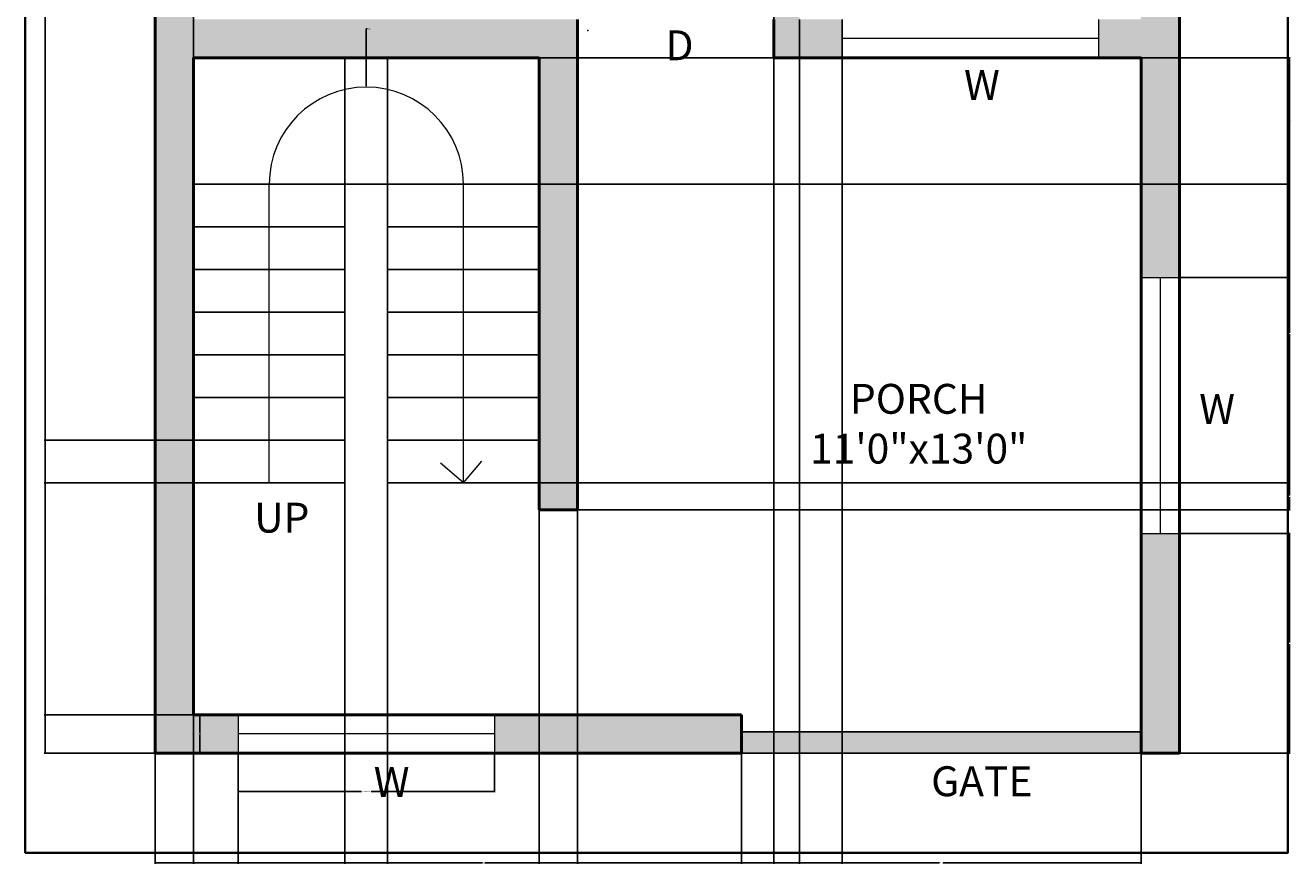
# Model space of a CAD drawing. Units: inches. Extents: x 1972 to 2269, y 1491 to 2023.
# Tile 1 of 3: x 1972 to 2269, y 1491 to 1687. Entities that reach past the tile are written whole.
import ezdxf

# ---------------------------------------------------------------- set-up
doc = ezdxf.new("R2010")
doc.units = ezdxf.units.IN
for name, color, linetype, lineweight in [('A-ANNO-DIMS', 2, 'Continuous', 18), ('A-ANNO-SYMB', 7, 'Continuous', 18), ('A-ANNO-TEXT', 7, 'Continuous', 18), ('A-ANNO-TTLB', 7, 'Continuous', 35), ('A-AREA-IDEN', 7, 'Continuous', 25), ('A-DOOR', 3, 'Continuous', 25), ('A-FLOR-STRS', 7, 'Continuous', 25), ('A-GLAZ', 4, 'Continuous', 18), ('A-WALL', 7, 'Continuous', 50)]:
    doc.layers.add(name, color=color, linetype=linetype, lineweight=lineweight)
doc.layers.add('A-DOOR-PATT', color=251, linetype='Continuous', lineweight=13, true_color=0x636466)
doc.layers.add('A-WALL-PATT', color=18, linetype='Continuous', lineweight=13, true_color=0x000000)
doc.styles.get("Standard").update_dxf_attribs({"font": 'arial.ttf'})
doc.dimstyles.get("Standard").update_dxf_attribs({"dimtxt": 0.18, "dimasz": 0.18, "dimexe": 0.18, "dimexo": 0.0625, "dimgap": 0.09, "dimtad": 0, "dimtih": 1, "dimtoh": 1, "dimdec": 4, "dimzin": 0, "dimdsep": 46, "dimtxsty": 'Standard', "dimcen": 0.09, "dimadec": 0, "dimazin": 0, "dimtfac": 1, "dimtdec": 4, "dimtofl": 0, "dimtmove": 0, "dimatfit": 3, "dimfxl": 1, "dimtolj": 1, "dimtzin": 0, "dimarcsym": 0})

# ---------------------------------------------------------------- blocks, each defined once
blk = doc.blocks.new('WINDOW-60IN')
for p, q in [((0, 60), (9, 60)), ((4.5, 60), (4.5, 0)), ((0, 0), (9, 0))]:
    blk.add_line(p, q)
blk = doc.blocks.new('*D12')
at = {"layer": 'A-ANNO-DIMS', "color": 0, "lineweight": -2, "transparency": 16777216}
for p, q in [((2022.33, 1516.54), (2022.33, 1507.42)), ((2082.33, 1516.54), (2082.33, 1507.42)), ((2022.51, 1507.6), (2051.21, 1507.6)), ((2082.15, 1507.6), (2053.44, 1507.6))]:
    blk.add_line(p, q, dxfattribs=at)
at = {"layer": 'A-ANNO-DIMS', "color": 0, "transparency": 16777216}
for points in [[(2022.51, 1507.63), (2022.51, 1507.57), (2022.33, 1507.6)], [(2082.15, 1507.63), (2082.15, 1507.57), (2082.33, 1507.6)]]:
    blk.add_solid(points, dxfattribs=at)
at = {"layer": 'Defpoints', "color": 0, "transparency": 16777216}
for p in [(2022.33, 1516.6), (2082.33, 1516.6), (2082.33, 1507.6)]:
    blk.add_point(p, dxfattribs=at)
at = {"layer": 'A-ANNO-DIMS', "color": 0, "transparency": 16777216, "insert": (2052.33, 1507.6), "char_height": 0.18, "attachment_point": 5}
blk.add_mtext('\\A1;WINDOW 60 TYP.', dxfattribs=at)
blk = doc.blocks.new('*D13')
at = {"layer": 'A-ANNO-DIMS', "color": 0, "lineweight": -2, "transparency": 16777216}
for p, q in [((2022.26, 1525.6), (2013.15, 1525.6)), ((2013.33, 1525.42), (2013.33, 1521.28)), ((2013.33, 1516.78), (2013.33, 1520.92)), ((2022.26, 1516.6), (2013.15, 1516.6))]:
    blk.add_line(p, q, dxfattribs=at)
at = {"layer": 'A-ANNO-DIMS', "color": 0, "transparency": 16777216}
for points in [[(2013.3, 1525.42), (2013.36, 1525.42), (2013.33, 1525.6)], [(2013.3, 1516.78), (2013.36, 1516.78), (2013.33, 1516.6)]]:
    blk.add_solid(points, dxfattribs=at)
at = {"layer": 'Defpoints', "color": 0, "transparency": 16777216}
for p in [(2022.33, 1525.6), (2013.33, 1516.6), (2022.33, 1516.6)]:
    blk.add_point(p, dxfattribs=at)
at = {"layer": 'A-ANNO-DIMS', "color": 0, "transparency": 16777216, "insert": (2013.33, 1521.1), "char_height": 0.18, "attachment_point": 5}
blk.add_mtext('\\A1;9 TYP.', dxfattribs=at)
blk = doc.blocks.new('*D29')
at = {"layer": 'A-ANNO-DIMS', "color": 0, "lineweight": -2, "transparency": 16777216}
for p, q in [((2002.76, 1996.6), (1976.9, 1996.6)), ((1977.08, 1996.42), (1977.08, 1756.78)), ((1977.08, 1516.78), (1977.08, 1756.42)), ((2002.76, 1516.6), (1976.9, 1516.6))]:
    blk.add_line(p, q, dxfattribs=at)
at = {"layer": 'A-ANNO-DIMS', "color": 0, "transparency": 16777216}
for points in [[(1977.05, 1996.42), (1977.11, 1996.42), (1977.08, 1996.6)], [(1977.05, 1516.78), (1977.11, 1516.78), (1977.08, 1516.6)]]:
    blk.add_solid(points, dxfattribs=at)
at = {"layer": 'Defpoints', "color": 0, "transparency": 16777216}
for p in [(1977.08, 1996.6), (2002.83, 1996.6), (2002.83, 1516.6)]:
    blk.add_point(p, dxfattribs=at)
at = {"layer": 'A-ANNO-DIMS', "color": 0, "transparency": 16777216, "insert": (1977.08, 1756.6), "char_height": 0.18, "attachment_point": 5}
blk.add_mtext('\\A1;480', dxfattribs=at)
blk = doc.blocks.new('*D30')
at = {"layer": 'A-ANNO-DIMS', "color": 0, "lineweight": -2, "transparency": 16777216}
for p, q in [((2233.89, 1679.6), (2268.76, 1679.6)), ((2268.58, 1679.42), (2268.58, 1654.03)), ((2268.58, 1628.28), (2268.58, 1653.67)), ((2242.89, 1628.1), (2268.76, 1628.1))]:
    blk.add_line(p, q, dxfattribs=at)
at = {"layer": 'A-ANNO-DIMS', "color": 0, "transparency": 16777216}
for points in [[(2268.55, 1679.42), (2268.61, 1679.42), (2268.58, 1679.6)], [(2268.55, 1628.28), (2268.61, 1628.28), (2268.58, 1628.1)]]:
    blk.add_solid(points, dxfattribs=at)
at = {"layer": 'Defpoints', "color": 0, "transparency": 16777216}
for p in [(2233.83, 1679.6), (2268.58, 1679.6), (2242.83, 1628.1)]:
    blk.add_point(p, dxfattribs=at)
at = {"layer": 'A-ANNO-DIMS', "color": 0, "transparency": 16777216, "insert": (2268.58, 1653.85), "char_height": 0.18, "attachment_point": 5}
blk.add_mtext('\\A1;51.5', dxfattribs=at)
blk = doc.blocks.new('*D36')
at = {"layer": 'A-ANNO-DIMS', "color": 0, "lineweight": -2, "transparency": 16777216}
for p, q in [((2242.89, 1568.1), (2268.76, 1568.1)), ((2268.58, 1567.92), (2268.58, 1542.53)), ((2268.58, 1516.78), (2268.58, 1542.17)), ((2242.89, 1516.6), (2268.76, 1516.6))]:
    blk.add_line(p, q, dxfattribs=at)
at = {"layer": 'A-ANNO-DIMS', "color": 0, "transparency": 16777216}
for points in [[(2268.55, 1567.92), (2268.61, 1567.92), (2268.58, 1568.1)], [(2268.55, 1516.78), (2268.61, 1516.78), (2268.58, 1516.6)]]:
    blk.add_solid(points, dxfattribs=at)
at = {"layer": 'Defpoints', "color": 0, "transparency": 16777216}
for p in [(2242.83, 1568.1), (2268.58, 1568.1), (2242.83, 1516.6)]:
    blk.add_point(p, dxfattribs=at)
at = {"layer": 'A-ANNO-DIMS', "color": 0, "transparency": 16777216, "insert": (2268.58, 1542.35), "char_height": 0.18, "attachment_point": 5}
blk.add_mtext('\\A1;51.5', dxfattribs=at)
blk = doc.blocks.new('*D37')
at = {"layer": 'A-ANNO-DIMS', "color": 0, "lineweight": -2, "transparency": 16777216}
for p, q in [((2153.83, 1688.54), (2153.83, 1490.67)), ((2163.83, 1688.54), (2163.83, 1490.67)), ((2154.01, 1490.85), (2158.62, 1490.85)), ((2163.65, 1490.85), (2159.04, 1490.85))]:
    blk.add_line(p, q, dxfattribs=at)
at = {"layer": 'A-ANNO-DIMS', "color": 0, "transparency": 16777216}
for points in [[(2154.01, 1490.88), (2154.01, 1490.82), (2153.83, 1490.85)], [(2163.65, 1490.88), (2163.65, 1490.82), (2163.83, 1490.85)]]:
    blk.add_solid(points, dxfattribs=at)
at = {"layer": 'Defpoints', "color": 0, "transparency": 16777216}
for p in [(2153.83, 1688.6), (2163.83, 1688.6), (2163.83, 1490.85)]:
    blk.add_point(p, dxfattribs=at)
at = {"layer": 'A-ANNO-DIMS', "color": 0, "transparency": 16777216, "insert": (2158.83, 1490.85), "char_height": 0.18, "attachment_point": 5}
blk.add_mtext('\\A1;10', dxfattribs=at)
blk = doc.blocks.new('*D40')
at = {"layer": 'A-ANNO-DIMS', "color": 0, "lineweight": -2, "transparency": 16777216}
for p, q in [((2002.83, 1516.54), (2002.83, 1490.67)), ((2022.33, 1516.54), (2022.33, 1490.67)), ((2003.01, 1490.85), (2012.26, 1490.85)), ((2022.15, 1490.85), (2012.89, 1490.85))]:
    blk.add_line(p, q, dxfattribs=at)
at = {"layer": 'A-ANNO-DIMS', "color": 0, "transparency": 16777216}
for points in [[(2003.01, 1490.88), (2003.01, 1490.82), (2002.83, 1490.85)], [(2022.15, 1490.88), (2022.15, 1490.82), (2022.33, 1490.85)]]:
    blk.add_solid(points, dxfattribs=at)
at = {"layer": 'Defpoints', "color": 0, "transparency": 16777216}
for p in [(2002.83, 1516.6), (2022.33, 1516.6), (2022.33, 1490.85)]:
    blk.add_point(p, dxfattribs=at)
at = {"layer": 'A-ANNO-DIMS', "color": 0, "transparency": 16777216, "insert": (2012.58, 1490.85), "char_height": 0.18, "attachment_point": 5}
blk.add_mtext('\\A1;19.5', dxfattribs=at)
blk = doc.blocks.new('*D41')
at = {"layer": 'A-ANNO-DIMS', "color": 0, "lineweight": -2, "transparency": 16777216}
for p, q in [((2140.25, 1521.54), (2140.25, 1490.67)), ((2233.83, 1521.54), (2233.83, 1490.67)), ((2140.43, 1490.85), (2186.64, 1490.85)), ((2233.65, 1490.85), (2187.43, 1490.85))]:
    blk.add_line(p, q, dxfattribs=at)
at = {"layer": 'A-ANNO-DIMS', "color": 0, "transparency": 16777216}
for points in [[(2140.43, 1490.88), (2140.43, 1490.82), (2140.25, 1490.85)], [(2233.65, 1490.88), (2233.65, 1490.82), (2233.83, 1490.85)]]:
    blk.add_solid(points, dxfattribs=at)
at = {"layer": 'Defpoints', "color": 0, "transparency": 16777216}
for p in [(2140.25, 1521.6), (2233.83, 1521.6), (2233.83, 1490.85)]:
    blk.add_point(p, dxfattribs=at)
at = {"layer": 'A-ANNO-DIMS', "color": 0, "transparency": 16777216, "insert": (2187.04, 1490.85), "char_height": 0.18, "attachment_point": 5}
blk.add_mtext('\\A1;93.58', dxfattribs=at)
blk = doc.blocks.new('*D42')
at = {"layer": 'A-ANNO-DIMS', "color": 0, "lineweight": -2, "transparency": 16777216}
for p, q in [((2101.83, 1679.54), (2101.83, 1490.67)), ((2147.83, 1679.54), (2147.83, 1490.67)), ((2102.01, 1490.85), (2124.6, 1490.85)), ((2147.65, 1490.85), (2125.05, 1490.85))]:
    blk.add_line(p, q, dxfattribs=at)
at = {"layer": 'A-ANNO-DIMS', "color": 0, "transparency": 16777216}
for points in [[(2102.01, 1490.88), (2102.01, 1490.82), (2101.83, 1490.85)], [(2147.65, 1490.88), (2147.65, 1490.82), (2147.83, 1490.85)]]:
    blk.add_solid(points, dxfattribs=at)
at = {"layer": 'Defpoints', "color": 0, "transparency": 16777216}
for p in [(2101.83, 1679.6), (2147.83, 1679.6), (2147.83, 1490.85)]:
    blk.add_point(p, dxfattribs=at)
at = {"layer": 'A-ANNO-DIMS', "color": 0, "transparency": 16777216, "insert": (2124.83, 1490.85), "char_height": 0.18, "attachment_point": 5}
blk.add_mtext('\\A1;46', dxfattribs=at)
blk = doc.blocks.new('*D45')
at = {"layer": 'A-ANNO-DIMS', "color": 0, "lineweight": -2, "transparency": 16777216}
for p, q in [((2011.83, 1579.9), (2011.83, 1490.67)), ((2047.33, 1579.9), (2047.33, 1490.67)), ((2012.01, 1490.85), (2029.25, 1490.85)), ((2047.15, 1490.85), (2029.9, 1490.85))]:
    blk.add_line(p, q, dxfattribs=at)
at = {"layer": 'A-ANNO-DIMS', "color": 0, "transparency": 16777216}
for points in [[(2012.01, 1490.88), (2012.01, 1490.82), (2011.83, 1490.85)], [(2047.15, 1490.88), (2047.15, 1490.82), (2047.33, 1490.85)]]:
    blk.add_solid(points, dxfattribs=at)
at = {"layer": 'Defpoints', "color": 0, "transparency": 16777216}
for p in [(2011.83, 1579.97), (2047.33, 1579.97), (2047.33, 1490.85)]:
    blk.add_point(p, dxfattribs=at)
at = {"layer": 'A-ANNO-DIMS', "color": 0, "transparency": 16777216, "insert": (2029.58, 1490.85), "char_height": 0.18, "attachment_point": 5}
blk.add_mtext('\\A1;35.5', dxfattribs=at)
blk = doc.blocks.new('*D46')
at = {"layer": 'A-ANNO-DIMS', "color": 0, "lineweight": -2, "transparency": 16777216}
for p, q in [((2047.33, 1579.9), (2047.33, 1490.67)), ((2057.33, 1579.9), (2057.33, 1490.67)), ((2047.51, 1490.85), (2052.12, 1490.85)), ((2057.15, 1490.85), (2052.54, 1490.85))]:
    blk.add_line(p, q, dxfattribs=at)
at = {"layer": 'A-ANNO-DIMS', "color": 0, "transparency": 16777216}
for points in [[(2047.51, 1490.88), (2047.51, 1490.82), (2047.33, 1490.85)], [(2057.15, 1490.88), (2057.15, 1490.82), (2057.33, 1490.85)]]:
    blk.add_solid(points, dxfattribs=at)
at = {"layer": 'Defpoints', "color": 0, "transparency": 16777216}
for p in [(2047.33, 1579.97), (2057.33, 1579.97), (2057.33, 1490.85)]:
    blk.add_point(p, dxfattribs=at)
at = {"layer": 'A-ANNO-DIMS', "color": 0, "transparency": 16777216, "insert": (2052.33, 1490.85), "char_height": 0.18, "attachment_point": 5}
blk.add_mtext('\\A1;10', dxfattribs=at)
blk = doc.blocks.new('*D47')
at = {"layer": 'A-ANNO-DIMS', "color": 0, "lineweight": -2, "transparency": 16777216}
for p, q in [((2092.89, 1649.97), (2268.76, 1649.97)), ((2268.58, 1649.79), (2268.58, 1615.15)), ((2268.58, 1580.15), (2268.58, 1614.78)), ((2092.89, 1579.97), (2268.76, 1579.97))]:
    blk.add_line(p, q, dxfattribs=at)
at = {"layer": 'A-ANNO-DIMS', "color": 0, "transparency": 16777216}
for points in [[(2268.55, 1649.79), (2268.61, 1649.79), (2268.58, 1649.97)], [(2268.55, 1580.15), (2268.61, 1580.15), (2268.58, 1579.97)]]:
    blk.add_solid(points, dxfattribs=at)
at = {"layer": 'Defpoints', "color": 0, "transparency": 16777216}
for p in [(2092.83, 1649.97), (2268.58, 1649.97), (2092.83, 1579.97)]:
    blk.add_point(p, dxfattribs=at)
at = {"layer": 'A-ANNO-DIMS', "color": 0, "transparency": 16777216, "insert": (2268.58, 1614.97), "char_height": 0.18, "attachment_point": 5}
blk.add_mtext('\\A1;70', dxfattribs=at)
blk = doc.blocks.new('*D48')
at = {"layer": 'A-ANNO-DIMS', "color": 0, "lineweight": -2, "transparency": 16777216}
for p, q in [((2092.89, 1679.6), (2268.76, 1679.6)), ((2268.58, 1679.42), (2268.58, 1664.96)), ((2268.58, 1650.15), (2268.58, 1664.6)), ((2092.89, 1649.97), (2268.76, 1649.97))]:
    blk.add_line(p, q, dxfattribs=at)
at = {"layer": 'A-ANNO-DIMS', "color": 0, "transparency": 16777216}
for points in [[(2268.55, 1679.42), (2268.61, 1679.42), (2268.58, 1679.6)], [(2268.55, 1650.15), (2268.61, 1650.15), (2268.58, 1649.97)]]:
    blk.add_solid(points, dxfattribs=at)
at = {"layer": 'Defpoints', "color": 0, "transparency": 16777216}
for p in [(2092.83, 1679.6), (2268.58, 1679.6), (2092.83, 1649.97)]:
    blk.add_point(p, dxfattribs=at)
at = {"layer": 'A-ANNO-DIMS', "color": 0, "transparency": 16777216, "insert": (2268.58, 1664.78), "char_height": 0.18, "attachment_point": 5}
blk.add_mtext('\\A1;29.63', dxfattribs=at)
blk = doc.blocks.new('*D49')
at = {"layer": 'A-ANNO-DIMS', "color": 0, "lineweight": -2, "transparency": 16777216}
for p, q in [((2011.76, 1589.97), (1976.9, 1589.97)), ((1977.08, 1589.79), (1977.08, 1585.15)), ((1977.08, 1580.15), (1977.08, 1584.78)), ((2011.76, 1579.97), (1976.9, 1579.97))]:
    blk.add_line(p, q, dxfattribs=at)
at = {"layer": 'A-ANNO-DIMS', "color": 0, "transparency": 16777216}
for points in [[(1977.05, 1589.79), (1977.11, 1589.79), (1977.08, 1589.97)], [(1977.05, 1580.15), (1977.11, 1580.15), (1977.08, 1579.97)]]:
    blk.add_solid(points, dxfattribs=at)
at = {"layer": 'Defpoints', "color": 0, "transparency": 16777216}
for p in [(1977.08, 1589.97), (2011.83, 1589.97), (2011.83, 1579.97)]:
    blk.add_point(p, dxfattribs=at)
at = {"layer": 'A-ANNO-DIMS', "color": 0, "transparency": 16777216, "insert": (1977.08, 1584.97), "char_height": 0.18, "attachment_point": 5}
blk.add_mtext('\\A1;10', dxfattribs=at)
blk = doc.blocks.new('*D50')
at = {"layer": 'A-ANNO-DIMS', "color": 0, "lineweight": -2, "transparency": 16777216}
for p, q in [((2092.83, 1573.54), (2092.83, 1490.67)), ((2101.83, 1573.54), (2101.83, 1490.67)), ((2093.01, 1490.85), (2097.18, 1490.85)), ((2101.65, 1490.85), (2097.48, 1490.85))]:
    blk.add_line(p, q, dxfattribs=at)
at = {"layer": 'A-ANNO-DIMS', "color": 0, "transparency": 16777216}
for points in [[(2093.01, 1490.88), (2093.01, 1490.82), (2092.83, 1490.85)], [(2101.65, 1490.88), (2101.65, 1490.82), (2101.83, 1490.85)]]:
    blk.add_solid(points, dxfattribs=at)
at = {"layer": 'Defpoints', "color": 0, "transparency": 16777216}
for p in [(2092.83, 1573.6), (2101.83, 1573.6), (2101.83, 1490.85)]:
    blk.add_point(p, dxfattribs=at)
at = {"layer": 'A-ANNO-DIMS', "color": 0, "transparency": 16777216, "insert": (2097.33, 1490.85), "char_height": 0.18, "attachment_point": 5}
blk.add_mtext('\\A1;9', dxfattribs=at)
blk = doc.blocks.new('*D51')
at = {"layer": 'A-ANNO-DIMS', "color": 0, "lineweight": -2, "transparency": 16777216}
for p, q in [((2011.76, 1579.97), (1976.9, 1579.97)), ((1977.08, 1579.79), (1977.08, 1552.96)), ((1977.08, 1525.78), (1977.08, 1552.6)), ((2011.76, 1525.6), (1976.9, 1525.6))]:
    blk.add_line(p, q, dxfattribs=at)
at = {"layer": 'A-ANNO-DIMS', "color": 0, "transparency": 16777216}
for points in [[(1977.05, 1579.79), (1977.11, 1579.79), (1977.08, 1579.97)], [(1977.05, 1525.78), (1977.11, 1525.78), (1977.08, 1525.6)]]:
    blk.add_solid(points, dxfattribs=at)
at = {"layer": 'Defpoints', "color": 0, "transparency": 16777216}
for p in [(1977.08, 1579.97), (2011.83, 1579.97), (2011.83, 1525.6)]:
    blk.add_point(p, dxfattribs=at)
at = {"layer": 'A-ANNO-DIMS', "color": 0, "transparency": 16777216, "insert": (1977.08, 1552.78), "char_height": 0.18, "attachment_point": 5}
blk.add_mtext('\\A1;54.37', dxfattribs=at)
blk = doc.blocks.new('*D56')
at = {"layer": 'A-ANNO-DIMS', "color": 0, "lineweight": -2, "transparency": 16777216}
for p, q in [((2011.83, 1832.54), (2011.83, 1490.67)), ((2147.83, 1796.54), (2147.83, 1490.67)), ((2012.01, 1490.85), (2079.55, 1490.85)), ((2147.65, 1490.85), (2080.11, 1490.85))]:
    blk.add_line(p, q, dxfattribs=at)
at = {"layer": 'A-ANNO-DIMS', "color": 0, "transparency": 16777216}
for points in [[(2012.01, 1490.88), (2012.01, 1490.82), (2011.83, 1490.85)], [(2147.65, 1490.88), (2147.65, 1490.82), (2147.83, 1490.85)]]:
    blk.add_solid(points, dxfattribs=at)
at = {"layer": 'Defpoints', "color": 0, "transparency": 16777216}
for p in [(2011.83, 1832.6), (2147.83, 1796.6), (2147.83, 1490.85)]:
    blk.add_point(p, dxfattribs=at)
at = {"layer": 'A-ANNO-DIMS', "color": 0, "transparency": 16777216, "insert": (2079.83, 1490.85), "char_height": 0.18, "attachment_point": 5}
blk.add_mtext('\\A1;136', dxfattribs=at)
blk = doc.blocks.new('*D58')
at = {"layer": 'A-ANNO-DIMS', "color": 0, "lineweight": -2, "transparency": 16777216}
for p, q in [((2092.89, 1579.97), (2268.76, 1579.97)), ((2268.58, 1579.79), (2268.58, 1576.96)), ((2268.58, 1573.78), (2268.58, 1576.6)), ((2092.89, 1573.6), (2268.76, 1573.6))]:
    blk.add_line(p, q, dxfattribs=at)
at = {"layer": 'A-ANNO-DIMS', "color": 0, "transparency": 16777216}
for points in [[(2268.55, 1579.79), (2268.61, 1579.79), (2268.58, 1579.97)], [(2268.55, 1573.78), (2268.61, 1573.78), (2268.58, 1573.6)]]:
    blk.add_solid(points, dxfattribs=at)
at = {"layer": 'Defpoints', "color": 0, "transparency": 16777216}
for p in [(2092.83, 1579.97), (2268.58, 1579.97), (2092.83, 1573.6)]:
    blk.add_point(p, dxfattribs=at)
at = {"layer": 'A-ANNO-DIMS', "color": 0, "transparency": 16777216, "insert": (2268.58, 1576.78), "char_height": 0.18, "attachment_point": 5}
blk.add_mtext('\\A1;6.367', dxfattribs=at)
blk = doc.blocks.new('*D62')
at = {"layer": 'A-ANNO-DIMS', "color": 0, "lineweight": -2, "transparency": 16777216}
for p, q in [((2124.71, 1712.14), (2117.13, 1702.46)), ((2124.89, 1712.14), (2124.71, 1712.14)), ((2104.13, 1685.96), (2104.31, 1685.96)), ((2104.22, 1685.87), (2104.22, 1686.05))]:
    blk.add_line(p, q, dxfattribs=at)
at = {"layer": 'A-ANNO-DIMS', "color": 0, "transparency": 16777216}
blk.add_solid([(2117.11, 1702.48), (2117.16, 1702.44), (2117.02, 1702.32)], dxfattribs=at)
at = {"layer": 'Defpoints', "color": 0, "transparency": 16777216}
for p in [(2117.02, 1702.32), (2104.22, 1685.96)]:
    blk.add_point(p, dxfattribs=at)
at = {"layer": 'A-ANNO-DIMS', "color": 0, "transparency": 16777216, "insert": (2125.63, 1712.14), "char_height": 0.18, "attachment_point": 5}
blk.add_mtext('\\A1;2X R20.778', dxfattribs=at)
blk = doc.blocks.new('*D63')
at = {"layer": 'A-ANNO-DIMS', "color": 0, "lineweight": -2, "transparency": 16777216}
for p, q in [((2052.51, 1686.37), (2052.33, 1686.37)), ((2052.33, 1686.37), (2052.33, 1672.9)), ((2052.24, 1649.97), (2052.42, 1649.97)), ((2052.33, 1649.88), (2052.33, 1650.06))]:
    blk.add_line(p, q, dxfattribs=at)
at = {"layer": 'A-ANNO-DIMS', "color": 0, "transparency": 16777216}
blk.add_solid([(2052.3, 1672.9), (2052.36, 1672.9), (2052.33, 1672.72)], dxfattribs=at)
at = {"layer": 'Defpoints', "color": 0, "transparency": 16777216}
for p in [(2052.33, 1672.72), (2052.33, 1649.97)]:
    blk.add_point(p, dxfattribs=at)
at = {"layer": 'A-ANNO-DIMS', "color": 0, "transparency": 16777216, "insert": (2052.99, 1686.37), "char_height": 0.18, "attachment_point": 5}
blk.add_mtext('\\A1;R22.75', dxfattribs=at)

msp = doc.modelspace()

# ---------------------------------------------------------------- hatches: boundary and pattern name
at = {"layer": 'A-DOOR-PATT'}
h = msp.add_hatch(color=256, dxfattribs=at)
h.dxf.hatch_style = 1
h.paths.add_polyline_path([(2233.8266, 1521.5987), (2140.2493, 1521.5987), (2140.2493, 1516.5987), (2233.8266, 1516.5987)])
at = {"layer": 'A-WALL-PATT'}
h = msp.add_hatch(color=256, dxfattribs=at)
h.dxf.hatch_style = 1
h.paths.add_polyline_path([(2242.8266, 1996.5987), (2002.8266, 1996.5987), (2002.8266, 1972.5987), (2011.8266, 1972.5987), (2011.8266, 1987.5987), (2092.8266, 1987.5987), (2101.8266, 1987.5987), (2233.8266, 1987.5987), (2233.8266, 1938.5987), (2242.8266, 1938.5987)])
h.paths.add_polyline_path([(2101.8266, 1957.5987, -0.08755883), (2092.8266, 1957.5987), (2092.8266, 1933.5987), (2011.8266, 1933.5987), (2011.8266, 1948.5987), (2002.8266, 1948.5987), (2002.8266, 1896.5987), (2011.8266, 1896.5987), (2011.8266, 1927.5987), (2092.8266, 1927.5987), (2092.8266, 1841.5987), (2041.8266, 1841.5987, -0.08755883), (2041.8266, 1832.5987), (2092.8266, 1832.5987), (2101.8266, 1832.5987), (2101.8266, 1868.5987)])
h.paths.add_polyline_path([(2242.8266, 1890.5987), (2233.8266, 1890.5987), (2233.8266, 1841.5987), (2137.8266, 1841.5987, -0.07106781), (2137.8266, 1832.5987), (2147.8266, 1832.5987), (2183.8266, 1832.5987), (2233.8266, 1832.5987), (2233.8266, 1790.5987), (2242.8266, 1790.5987)])
h.paths.add_polyline_path([(2011.8266, 1832.5987), (2011.8266, 1862.5987), (2011.8266, 1872.5987), (2002.8266, 1872.5987), (2002.8266, 1516.5987), (2022.3266, 1516.5987), (2022.3266, 1525.5987), (2011.8266, 1525.5987), (2011.8266, 1679.5987), (2092.8266, 1679.5987), (2092.8266, 1643.5987), (2092.8266, 1573.5987), (2101.8266, 1573.5987), (2101.8266, 1643.5987), (2101.8266, 1679.5987), (2101.8266, 1688.5987), (2011.8266, 1688.5987)])
h.paths.add_polyline_path([(2140.2493, 1525.5987), (2101.8266, 1525.5987), (2092.8266, 1525.5987), (2082.3266, 1525.5987), (2082.3266, 1516.5987), (2140.2493, 1516.5987)])
h.paths.add_polyline_path([(2242.8266, 1568.0987), (2233.8266, 1568.0987), (2233.8266, 1525.5987), (2233.8266, 1516.5987), (2242.8266, 1516.5987)])
h.paths.add_polyline_path([(2242.8266, 1730.5987), (2233.8266, 1730.5987), (2233.8266, 1688.5987), (2223.8266, 1688.5987), (2223.8266, 1679.5987), (2233.8266, 1679.5987), (2233.8266, 1628.0987), (2242.8266, 1628.0987)])
h.paths.add_polyline_path([(2163.8266, 1688.5987), (2153.8266, 1688.5987), (2153.8266, 1796.5987, -0.04536102), (2147.8266, 1796.5987), (2147.8266, 1688.5987), (2147.8266, 1679.5987), (2153.8266, 1679.5987), (2163.8266, 1679.5987)])

# ---------------------------------------------------------------- linework, layer by layer
at = {"layer": 'A-ANNO-SYMB'}
for p, q in [((2029.5766, 1579.9658), (2029.5766, 1649.9658)), ((2075.0766, 1579.9658), (2075.0766, 1649.9658)), ((2075.0766, 1579.9658), (2069.7273, 1584.527)), ((2075.0766, 1579.9658), (2079.4235, 1585.0639))]:
    msp.add_line(p, q, dxfattribs=at)
msp.add_arc((2052.3266, 1649.9658), 22.75, 360, 180, dxfattribs=at)
at = {"layer": 'A-ANNO-TTLB'}
msp.add_lwpolyline([(1972.4438, 2012.9515), (2268.2203, 2012.9515), (2268.2203, 1493.2355), (1972.4438, 1493.2355)], close=True, dxfattribs=at)
at = {"layer": 'A-DOOR'}
for p, q in [((2140.2493, 1521.5987), (2233.8266, 1521.5987)), ((2140.2493, 1516.5987), (2233.8266, 1516.5987))]:
    msp.add_line(p, q, dxfattribs=at)
at = {"layer": 'A-FLOR-STRS'}
for p, q in [((2047.3266, 1679.5987), (2047.3266, 1579.9658)), ((2057.3266, 1679.5987), (2057.3266, 1579.9658)), ((2011.8266, 1649.9658), (2092.8266, 1649.9658)), ((2011.8266, 1639.9658), (2047.3266, 1639.9658)), ((2057.3266, 1639.9658), (2092.8266, 1639.9658)), ((2011.8266, 1629.9658), (2047.3266, 1629.9658)), ((2057.3266, 1629.9658), (2092.8266, 1629.9658)), ((2011.8266, 1619.9658), (2047.3266, 1619.9658)), ((2057.3266, 1619.9658), (2092.8266, 1619.9658)), ((2011.8266, 1609.9658), (2047.3266, 1609.9658)), ((2057.3266, 1609.9658), (2092.8266, 1609.9658)), ((2011.8266, 1599.9658), (2047.3266, 1599.9658)), ((2057.3266, 1599.9658), (2092.8266, 1599.9658)), ((2011.8266, 1589.9658), (2047.3266, 1589.9658)), ((2057.3266, 1589.9658), (2092.8266, 1589.9658)), ((2011.8266, 1579.9658), (2047.3266, 1579.9658)), ((2057.3266, 1579.9658), (2092.8266, 1579.9658))]:
    msp.add_line(p, q, dxfattribs=at)
at = {"layer": 'A-WALL'}
for p, q in [((2002.8266, 1516.5987), (2002.8266, 1996.5987)), ((2242.8266, 1996.5987), (2242.8266, 1516.5987)), ((2101.8266, 1679.5987), (2101.8266, 1688.5987)), ((2147.8266, 1688.5987), (2147.8266, 1679.5987)), ((2011.8266, 1525.5987), (2011.8266, 1679.5987)), ((2092.8266, 1679.5987), (2011.8266, 1679.5987)), ((2092.8266, 1643.5987), (2092.8266, 1679.5987)), ((2101.8266, 1643.5987), (2101.8266, 1679.5987)), ((2153.8266, 1679.5987), (2147.8266, 1679.5987)), ((2153.8266, 1679.5987), (2233.8266, 1679.5987)), ((2233.8266, 1679.5987), (2233.8266, 1516.5987)), ((2011.8266, 1525.5987), (2011.8266, 1643.5987)), ((2092.8266, 1643.5987), (2092.8266, 1573.5987)), ((2101.8266, 1643.5987), (2101.8266, 1573.5987)), ((2233.8266, 1643.5987), (2233.8266, 1525.5987)), ((2092.8266, 1573.5987), (2101.8266, 1573.5987)), ((2092.8266, 1525.5987), (2011.8266, 1525.5987)), ((2092.8266, 1525.5987), (2101.8266, 1525.5987)), ((2140.2493, 1525.5987), (2101.8266, 1525.5987)), ((2140.2493, 1525.5987), (2101.8266, 1525.5987)), ((2140.2493, 1525.5987), (2140.2493, 1516.5987)), ((2233.8266, 1525.5987), (2233.8266, 1516.5987)), ((2140.2493, 1516.5987), (2002.8266, 1516.5987)), ((2242.8266, 1516.5987), (2233.8266, 1516.5987))]:
    msp.add_line(p, q, dxfattribs=at)

# ---------------------------------------------------------------- block references
at = {"layer": 'A-GLAZ'}
for p, rotation in [((2163.8268, 1688.5983), 270.0000000000006), ((2022.3268, 1525.5983), 270.0000000000001)]:
    msp.add_blockref('WINDOW-60IN', p, dxfattribs=dict(at, rotation=rotation))
msp.add_blockref('WINDOW-60IN', (2233.827, 1568.099), dxfattribs=at)

# ---------------------------------------------------------------- texts
at = {"layer": 'A-ANNO-TEXT', "char_height": 7, "attachment_point": 1}
for s, width, insert in [('\\pxqc;D', 10.77063, (2120.3238, 1686.018)), ('\\pxqc;W', 19.209889, (2186.9391, 1676.7298)), ('\\pxqc;W', 23.220679, (2240.0281, 1600.7654)), ('\\pxqc;{\\fArial|b1|i0|c0|p34;UP}', 20.14067, (2022.4502, 1575.2844)), ('\\pxqc;W', 19.648624, (2048.433, 1513.3423)), ('\\pxqc;{\\fArial|b1|i0|c0|p34;GATE}', 32.875326, (2180.0755, 1513.4963))]:
    msp.add_mtext_dynamic_manual_height_columns(s, width=width, gutter_width=12.5, heights=[0], dxfattribs=dict(at, insert=insert))
at = {"layer": 'A-AREA-IDEN', "insert": (2144.3802, 1603.1397), "char_height": 7, "attachment_point": 1}
msp.add_mtext_dynamic_manual_height_columns('\\pxqc;{\\fArial|b1|i0|c0|p34;PORCH\\P11\'0"x13\'0"}', width=74.737134, gutter_width=12.5, heights=[0], dxfattribs=at)

# ---------------------------------------------------------------- dimensions: what is measured, and where the dimension line sits
at = {"layer": 'A-ANNO-DIMS'}
for base, p1, p2, override, picture, middle in [((1977.0766, 1996.5987), (2002.8266, 1516.5987), (2002.8266, 1996.5987), {"dimdec": 0, "dimlfac": 1, "dimrnd": 0, "dimzin": 0, "dimdsep": 46, "dimlunit": 2}, '*D29', (1977.0766, 1756.5987)), ((2268.5766, 1679.5987), (2092.8266, 1649.9658), (2092.8266, 1679.5987), {"dimdec": 2, "dimlfac": 1, "dimrnd": 0, "dimzin": 0, "dimdsep": 46, "dimlunit": 2}, '*D48', (2268.5766, 1664.7823)), ((2268.5766, 1679.5987), (2242.8266, 1628.0987), (2233.8266, 1679.5987), {"dimdec": 1, "dimlfac": 1, "dimrnd": 0, "dimzin": 0, "dimdsep": 46, "dimlunit": 2}, '*D30', (2268.5766, 1653.8487)), ((2268.5766, 1649.9658), (2092.8266, 1579.9658), (2092.8266, 1649.9658), {"dimdec": 0, "dimlfac": 1, "dimrnd": 0, "dimzin": 0, "dimdsep": 46, "dimlunit": 2}, '*D47', (2268.5766, 1614.9658)), ((1977.0766, 1589.9658), (2011.8266, 1579.9658), (2011.8266, 1589.9658), {"dimdec": 0, "dimlfac": 1, "dimrnd": 0, "dimzin": 0, "dimdsep": 46, "dimlunit": 2}, '*D49', (1977.0766, 1584.9658)), ((1977.0766, 1579.9658), (2011.8266, 1525.5987), (2011.8266, 1579.9658), {"dimdec": 2, "dimlfac": 1, "dimrnd": 0, "dimzin": 0, "dimdsep": 46, "dimlunit": 2}, '*D51', (1977.0766, 1552.7823)), ((2268.5766, 1579.9658), (2092.8266, 1573.5987), (2092.8266, 1579.9658), {"dimdec": 3, "dimlfac": 1, "dimrnd": 0, "dimzin": 0, "dimdsep": 46, "dimlunit": 2}, '*D58', (2268.5766, 1576.7823)), ((2268.5766, 1568.0987), (2242.8266, 1516.5987), (2242.8266, 1568.0987), {"dimdec": 1, "dimlfac": 1, "dimrnd": 0, "dimzin": 0, "dimdsep": 46, "dimlunit": 2}, '*D36', (2268.5766, 1542.3487))]:
    dim = msp.add_linear_dim(base=base, p1=p1, p2=p2, angle=90, dimstyle='Standard', override=override, dxfattribs=at)
    dim.commit()
    dim.dimension.update_dxf_attribs({"geometry": picture, "text_midpoint": middle})
for base, p1, p2, override, picture, middle in [((2147.8266, 1490.8487), (2011.8266, 1832.5987), (2147.8266, 1796.5987), {"dimdec": 0, "dimlfac": 1, "dimrnd": 0, "dimzin": 0, "dimdsep": 46, "dimlunit": 2}, '*D56', (2079.8266, 1490.8487)), ((2163.8266, 1490.8487), (2153.8266, 1688.5987), (2163.8266, 1688.5987), {"dimdec": 0, "dimlfac": 1, "dimrnd": 0, "dimzin": 0, "dimdsep": 46, "dimlunit": 2}, '*D37', (2158.8266, 1490.8487)), ((2147.8266, 1490.8487), (2101.8266, 1679.5987), (2147.8266, 1679.5987), {"dimdec": 0, "dimlfac": 1, "dimrnd": 0, "dimzin": 0, "dimdsep": 46, "dimlunit": 2}, '*D42', (2124.8266, 1490.8487)), ((2047.3266, 1490.8487), (2011.8266, 1579.9658), (2047.3266, 1579.9658), {"dimdec": 1, "dimlfac": 1, "dimrnd": 0, "dimzin": 0, "dimdsep": 46, "dimlunit": 2}, '*D45', (2029.5766, 1490.8487)), ((2057.3266, 1490.8487), (2047.3266, 1579.9658), (2057.3266, 1579.9658), {"dimdec": 0, "dimlfac": 1, "dimrnd": 0, "dimzin": 0, "dimdsep": 46, "dimlunit": 2}, '*D46', (2052.3266, 1490.8487)), ((2101.8266, 1490.8487), (2092.8266, 1573.5987), (2101.8266, 1573.5987), {"dimdec": 0, "dimlfac": 1, "dimrnd": 0, "dimzin": 0, "dimdsep": 46, "dimlunit": 2}, '*D50', (2097.3266, 1490.8487)), ((2233.8266, 1490.8487), (2140.2493, 1521.5987), (2233.8266, 1521.5987), {"dimdec": 2, "dimlfac": 1, "dimrnd": 0, "dimzin": 0, "dimdsep": 46, "dimlunit": 2}, '*D41', (2187.0379, 1490.8487)), ((2022.3266, 1490.8487), (2002.8266, 1516.5987), (2022.3266, 1516.5987), {"dimdec": 1, "dimlfac": 1, "dimrnd": 0, "dimzin": 0, "dimdsep": 46, "dimlunit": 2}, '*D40', (2012.5766, 1490.8487))]:
    dim = msp.add_linear_dim(base=base, p1=p1, p2=p2, dimstyle='Standard', override=override, dxfattribs=at)
    dim.commit()
    dim.dimension.update_dxf_attribs({"geometry": picture, "text_midpoint": middle})
dim = msp.add_radius_dim(center=(2104.2173, 1685.9591), mpoint=(2117.0227, 1702.3216), text='2X <>', dimstyle='Standard', override={"dimdec": 3, "dimlfac": 1, "dimrnd": 0, "dimzin": 0, "dimdsep": 46, "dimlunit": 2}, dxfattribs=at)
dim.commit()
dim.dimension.update_dxf_attribs({"geometry": '*D62', "text_midpoint": (2125.6308, 1712.1391), "dimtype": 164})
dim = msp.add_radius_dim(center=(2052.3266, 1649.9658), mpoint=(2052.327, 1672.7158), dimstyle='Standard', override={"dimdec": 2, "dimlfac": 1, "dimrnd": 0, "dimzin": 0, "dimdsep": 46, "dimlunit": 2}, dxfattribs=at)
dim.commit()
dim.dimension.update_dxf_attribs({"geometry": '*D63', "text_midpoint": (2052.9878, 1686.3658), "dimtype": 164})
dim = msp.add_linear_dim(base=(2013.3266, 1516.5987), p1=(2022.3266, 1525.5987), p2=(2022.3266, 1516.5987), angle=270, text='<> TYP.', dimstyle='Standard', override={"dimdec": 0, "dimlfac": 1, "dimrnd": 0, "dimzin": 0, "dimdsep": 46, "dimlunit": 2}, dxfattribs=at)
dim.commit()
dim.dimension.update_dxf_attribs({"geometry": '*D13', "text_midpoint": (2013.3266, 1521.0987)})
dim = msp.add_linear_dim(base=(2082.3266, 1507.5987), p1=(2022.3266, 1516.5987), p2=(2082.3266, 1516.5987), text='WINDOW <> TYP.', dimstyle='Standard', override={"dimdec": 0, "dimlfac": 1, "dimrnd": 0, "dimzin": 0, "dimdsep": 46, "dimlunit": 2}, dxfattribs=at)
dim.commit()
dim.dimension.update_dxf_attribs({"geometry": '*D12', "text_midpoint": (2052.3266, 1507.5987)})

doc.saveas('drawing.dxf')
